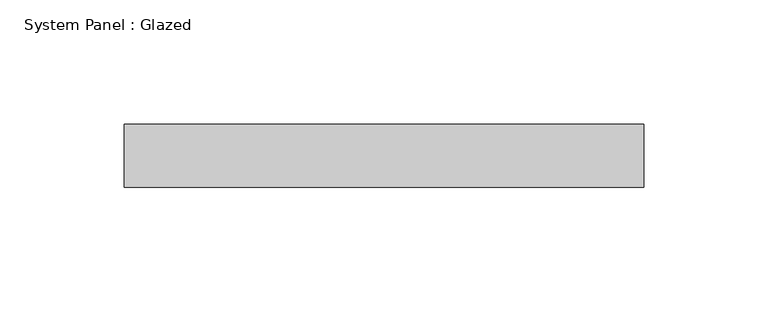
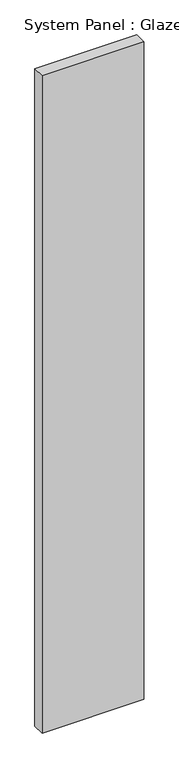
"""IFC4 building model written with IfcOpenShell, lengths in millimetres: plate geometry, System Panel : Glazed."""

from ifc_helpers import new_model, si_unit, origin, origin_with_axes, place, context, project, spatial, polyline, outline, extrude, source, transform, mapped, element, save


def system_panel_glazed_a4d46631(model_context):
    return source(origin(), model_context, "Body", "SweptSolid", [
        extrude(outline(polyline([(104.775, 19.05), (-104.775, 19.05), (-104.775, 44.45), (104.775, 44.45), (104.775, 19.05)])), origin_with_axes(), (0.0, 0.0, 1.0), 1428.75),
    ])


if __name__ == "__main__":
    model = new_model("IFC4")
    model_context = context("Model", 3, world=origin())
    ifc_project = project(units=[si_unit("LENGTHUNIT", "METRE", prefix="MILLI")], contexts=[model_context])
    site = spatial("IfcSite", under=ifc_project)
    building = spatial("IfcBuilding", under=site)
    placement = place(None, origin())
    system_panel_glazed_shape = system_panel_glazed_a4d46631(model_context)
    element("IfcPlate", 1, ObjectType="System Panel : Glazed", at=placement, inside=building, context=model_context, shape_type="MappedRepresentation", body=[
        mapped(system_panel_glazed_shape, transform((0.0, 0.0, 0.0), x_axis=(1.0, 0.0, 0.0), y_axis=(0.0, 1.0, 0.0), z_axis=(0.0, 0.0, 1.0))),
    ])
    save(model, "model.ifc")

# Revit data of these elements
# Type "System Panel : Glazed"
#   Construction Type Id = "GSP4R"
#   Analytic Construction = "1/8 in Pilkington single glazing"
#   Visual Light Transmittance = 0.9
#   Solar Heat Gain Coefficient = 0.86
#   Heat Transfer Coefficient (U) = 1.18115 BTU/(h·ft²·°F)
#   Define Thermal Properties by = 1
# Element 1 (IfcPlate, "System Panel : Glazed")
#   Materials on its faces: "Glass"
# Materials
#   "Glass": class "Glass", colour RGB 0 128 192, transparency 0.75, Description = "Soda Lime Glass", Cost = 0
